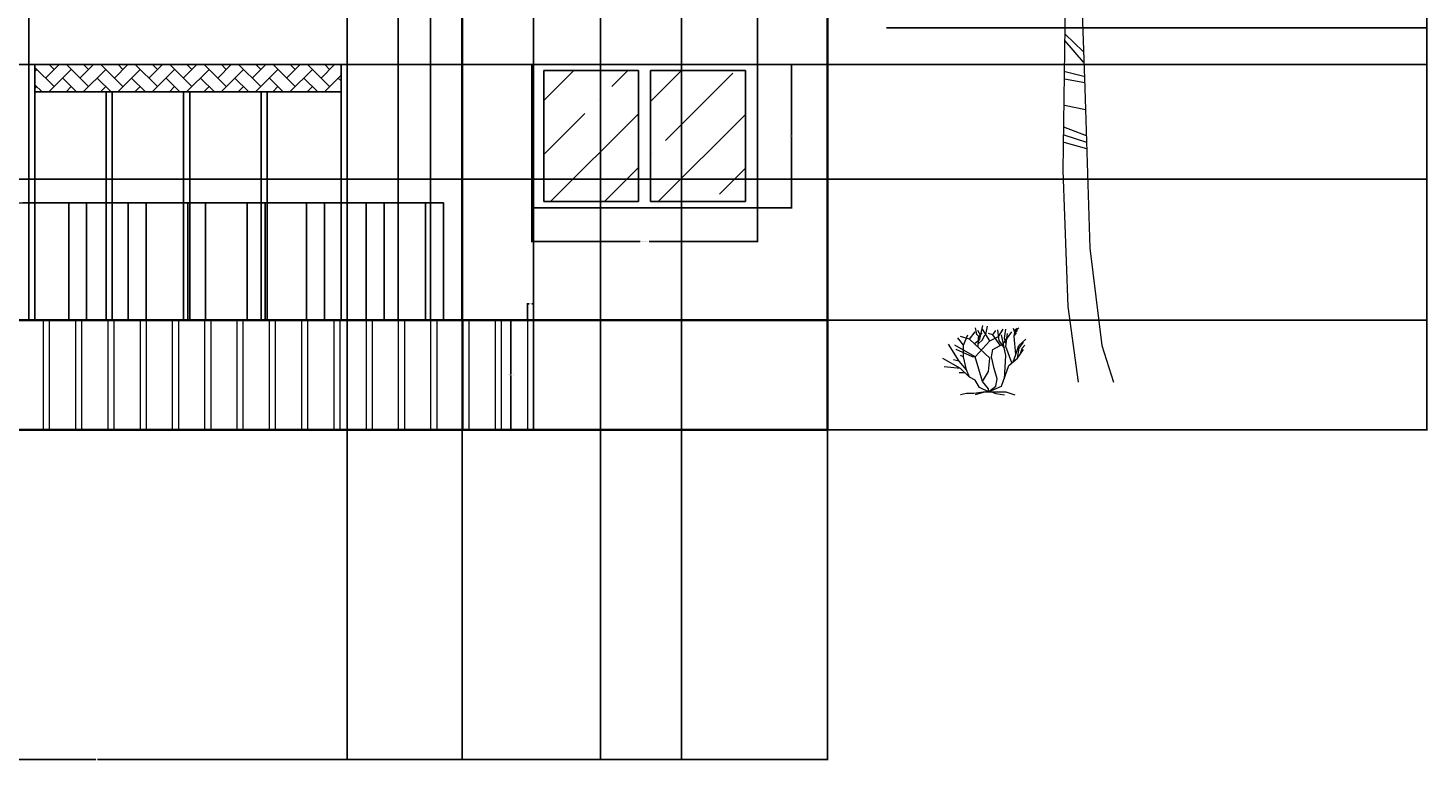
# Model space of a CAD drawing. Units: inches. Extents: x -177 to 697, y -125 to 346.
# Tile 3 of 4: x 237 to 697, y -125 to 116. Entities that reach past the tile are written whole.
import ezdxf

# ---------------------------------------------------------------- set-up
doc = ezdxf.new("R2010")
doc.units = ezdxf.units.IN
doc.header["$MEASUREMENT"] = 0
for name, color, linetype, lineweight in [('A-ANNO-DIMS', 2, 'Continuous', 18), ('A-DOOR', 3, 'Continuous', 25), ('A-FLOR-DECK', 8, 'Continuous', 18), ('A-FLOR-HRAL', 2, 'Continuous', 25), ('A-GLAZ', 4, 'Continuous', 25), ('A-GLAZ-PATT', 252, 'Continuous', 13), ('A-WALL', 7, 'Continuous', 35), ('L-PLNT', 94, 'Continuous', 13), ('S-FNDN', 7, 'Continuous', 35)]:
    doc.layers.add(name, color=color, linetype=linetype, lineweight=lineweight)
doc.styles.get("Standard").update_dxf_attribs({"font": 'arial.ttf'})
doc.dimstyles.get("Standard").update_dxf_attribs({"dimtxt": 0.18, "dimasz": 0.18, "dimexe": 0.18, "dimexo": 0.0625, "dimgap": 0.09, "dimtad": 0, "dimtih": 1, "dimtoh": 1, "dimdec": 4, "dimzin": 0, "dimdsep": 46, "dimtxsty": 'Standard', "dimcen": 0.09, "dimadec": 0, "dimazin": 0, "dimtfac": 1, "dimtdec": 4, "dimtofl": 0, "dimtmove": 0, "dimatfit": 3, "dimfxl": 1, "dimtolj": 1, "dimtzin": 0, "dimarcsym": 0})

# ---------------------------------------------------------------- blocks, each defined once
blk = doc.blocks.new('*U2')
for p, q in [((-7.5, 199.68), (-7.5, 197.946)), ((-5.567, 196.707), (-4.987, 201.167)), ((-4.407, 195.716), (-3.247, 200.672)), ((-2.474, 193.733), (-1.315, 199.433)), ((15.116, 194.477), (17.822, 198.689)), ((18.015, 195.716), (20.914, 198.689)), ((21.301, 196.459), (22.847, 198.441)), ((-20.064, 191.751), (-25.863, 193.238)), ((-15.232, 191.255), (-20.644, 193.981)), ((-9.433, 189.025), (-15.618, 193.238)), ((-6.727, 197.202), (-11.366, 197.45)), ((-3.441, 194.477), (-10.013, 195.716)), ((-1.894, 192.494), (-9.24, 193.733)), ((-1.121, 190.759), (0.232, 196.955)), ((0.038, 188.281), (1.778, 193.981)), ((5.837, 187.786), (7.577, 194.229)), ((9.317, 191.255), (10.283, 196.955)), ((11.829, 192.99), (13.182, 197.45)), ((13.956, 194.229), (14.729, 196.955)), ((14.536, 193.981), (17.242, 191.255)), ((16.082, 194.972), (17.822, 192.494)), ((18.015, 195.468), (18.981, 192.494)), ((19.368, 196.459), (19.948, 193.733)), ((20.914, 196.459), (21.301, 194.972)), ((22.074, 196.707), (23.427, 195.716)), ((23.234, 196.707), (23.62, 197.698)), ((-29.729, 190.759), (-31.469, 191.255)), ((-30.309, 190.512), (-30.695, 189.025)), ((-25.283, 191.751), (-29.342, 192.246)), ((-28.763, 190.759), (-28.763, 188.281)), ((-26.443, 191.503), (-26.636, 186.051)), ((-23.737, 191.751), (-24.51, 185.06)), ((-21.031, 191.998), (-21.804, 183.325)), ((-17.551, 191.503), (-20.451, 181.343)), ((-14.265, 190.759), (-18.131, 182.086)), ((-11.753, 189.768), (-15.425, 182.83)), ((-6.147, 186.299), (-9.24, 190.264)), ((-0.541, 189.52), (-7.307, 192.494)), ((-5.76, 190.016), (0.618, 185.308)), ((1.005, 185.803), (2.358, 190.759)), ((4.098, 185.06), (4.678, 190.512)), ((8.544, 190.512), (13.763, 189.52)), ((11.25, 192.494), (15.889, 190.512)), ((15.695, 186.299), (19.368, 188.777)), ((19.368, 187.29), (26.133, 189.768)), ((24.78, 187.538), (31.546, 188.777)), ((-8.08, 188.034), (-12.912, 182.83)), ((-4.987, 185.803), (-10.979, 182.086)), ((-5.76, 188.034), (-1.508, 182.582)), ((-2.668, 185.803), (1.198, 181.343)), ((1.005, 182.582), (2.938, 186.547)), ((4.871, 186.051), (10.09, 186.547)), ((4.871, 181.591), (8.544, 184.812)), ((6.997, 188.529), (12.216, 187.786)), ((9.51, 184.317), (15.502, 188.034)), ((11.25, 184.812), (17.628, 180.352)), ((14.536, 185.803), (19.948, 180.847)), ((17.242, 186.547), (23.041, 180.599)), ((20.721, 187.042), (25.167, 181.343)), ((23.814, 187.29), (26.907, 181.343)), ((26.133, 187.29), (29.419, 181.838)), ((28.066, 187.29), (30.966, 182.582)), ((29.806, 186.795), (32.319, 183.078)), ((29.999, 186.795), (33.092, 187.29)), ((32.512, 186.299), (35.218, 186.299)), ((33.479, 186.051), (34.445, 182.83)), ((35.605, 185.556), (37.151, 185.308)), ((35.798, 185.308), (36.958, 181.591)), ((38.118, 184.317), (38.504, 181.838)), ((-15.618, 179.36), (-20.644, 178.617)), ((-15.038, 179.36), (-10.786, 174.404)), ((-12.332, 180.104), (-9.433, 175.643)), ((-10.206, 180.104), (-8.08, 175.891)), ((-8.273, 180.104), (-6.147, 176.635)), ((-3.247, 183.821), (-8.08, 181.838)), ((-6.34, 179.608), (-4.6, 177.13)), ((-1.315, 181.591), (-5.374, 181.095)), ((-4.021, 179.36), (-2.861, 177.378)), ((-0.348, 180.352), (-1.894, 180.104)), ((2.938, 182.582), (6.61, 183.821)), ((4.098, 180.847), (8.35, 179.608)), ((5.644, 181.838), (13.569, 178.865)), ((7.384, 178.369), (10.476, 179.36)), ((7.77, 183.325), (16.082, 179.856)), ((39.857, 182.83), (40.244, 181.591)), ((-25.09, 175.148), (-28.376, 174.404)), ((-21.031, 177.626), (-24.897, 176.387)), ((-24.317, 175.891), (-18.711, 168.457)), ((-22.191, 176.635), (-16.391, 169.448)), ((-20.064, 177.626), (-15.812, 172.67)), ((-17.358, 178.617), (-13.299, 173.661)), ((-4.214, 175.148), (-14.072, 170.935)), ((-1.701, 176.882), (-8.66, 175.396)), ((-4.6, 174.9), (-4.021, 166.722)), ((-2.668, 176.387), (-2.376, 170.594)), ((-0.928, 176.882), (-1.508, 173.909)), ((2.551, 175.891), (-0.928, 171.431)), ((1.585, 177.13), (0.038, 174.652)), ((1.585, 177.13), (6.61, 176.139)), ((2.938, 175.891), (8.737, 173.413)), ((6.224, 178.121), (8.157, 175.148)), ((8.157, 178.121), (10.476, 172.422)), ((10.476, 177.874), (12.796, 169.696)), ((11.829, 177.874), (18.015, 179.113)), ((13.182, 177.874), (14.729, 166.97)), ((15.889, 177.13), (16.855, 164.492)), ((18.015, 177.13), (26.133, 179.113)), ((18.981, 175.891), (19.561, 163.005)), ((20.914, 175.891), (30.966, 176.635)), ((21.688, 175.396), (22.074, 161.518)), ((-28.956, 172.174), (-32.435, 170.192)), ((-27.409, 173.413), (-30.695, 172.67)), ((-29.922, 170.687), (-27.989, 165.235)), ((-27.989, 172.422), (-26.056, 166.227)), ((-26.829, 173.661), (-23.544, 167.218)), ((-25.476, 174.652), (-21.224, 167.466)), ((-8.466, 171.678), (-16.585, 167.713)), ((-8.853, 170.935), (-7.113, 160.527)), ((-6.92, 172.917), (-5.374, 163.253)), ((3.711, 174.404), (-0.541, 167.961)), ((5.257, 171.926), (-0.155, 163.005)), ((4.291, 173.909), (12.216, 168.953)), ((6.417, 170.439), (14.729, 164.492)), ((23.814, 174.404), (25.554, 160.279)), ((25.554, 173.661), (33.285, 173.661)), ((26.52, 173.165), (28.066, 159.784)), ((28.839, 172.174), (36.378, 170.687)), ((29.226, 171.926), (30.966, 158.545)), ((30.966, 170.687), (38.891, 167.713)), ((-32.628, 167.961), (-33.208, 167.961)), ((-32.628, 167.713), (-32.435, 165.979)), ((-31.082, 169.944), (-32.435, 169.2)), ((-31.662, 168.705), (-31.082, 165.483)), ((-12.139, 167.961), (-19.098, 162.014)), ((-12.719, 166.722), (-9.046, 154.828)), ((-10.979, 168.457), (-7.887, 157.801)), ((7.384, 168.705), (0.812, 157.553)), ((8.544, 165.979), (16.662, 160.527)), ((32.126, 169.696), (32.512, 158.545)), ((34.058, 168.705), (34.445, 158.545)), ((35.412, 167.713), (41.404, 164.988)), ((36.378, 166.474), (35.605, 158.792)), ((-14.265, 164.244), (-19.678, 158.049)), ((-14.265, 163.749), (-10.786, 154.828)), ((9.317, 164.244), (2.358, 154.332)), ((10.09, 162.51), (17.435, 157.058)), ((37.731, 165.235), (36.958, 159.288)), ((37.924, 165.235), (41.404, 163.749)), ((38.504, 164.492), (38.504, 159.536)), ((39.664, 163.253), (42.37, 161.766)), ((39.857, 162.757), (39.857, 160.031)), ((40.824, 161.766), (41.21, 160.031)), ((41.21, 161.518), (42.757, 160.279)), ((-16.005, 160.031), (-19.484, 154.084)), ((-16.585, 158.545), (-13.106, 152.35)), ((-15.618, 160.775), (-12.332, 154.332)), ((10.863, 159.784), (4.484, 152.35)), ((11.443, 157.553), (16.855, 154.332)), ((-18.131, 153.589), (-19.484, 151.606)), ((-17.938, 152.597), (-16.972, 151.111)), ((-17.358, 155.819), (-14.845, 151.358)), ((11.829, 155.075), (6.804, 150.119)), ((12.216, 153.093), (16.082, 151.606)), ((12.603, 151.111), (8.544, 148.385)), ((12.216, 148.137), (10.09, 147.393)), ((12.603, 149.872), (15.116, 149.128)), ((12.409, 145.659), (11.056, 145.659)), ((12.409, 146.898), (13.763, 146.402)), ((-4.081, 140.645), (0.753, 138.261)), ((-4.081, 137.547), (0.753, 135.163)), ((-4.081, 129.205), (1.124, 126.821)), ((-4.081, 127.298), (1.31, 123.246)), ((-4.081, 121.578), (1.31, 120.863)), ((-4.453, 112.283), (1.682, 105.133)), ((-4.267, 114.428), (1.682, 108.708)), ((-4.639, 102.273), (1.868, 100.604)), ((-4.453, 99.651), (2.24, 98.459)), ((-4.453, 91.071), (2.426, 89.641)), ((-4.825, 83.921), (2.612, 81.061)), ((-4.639, 81.299), (2.797, 78.916)), ((-4.639, 78.916), (2.797, 76.771))]:
    blk.add_line(p, q)
for points in [[(-2.363, 170.553), (-3.88, 148.505), (-4.988, 69.634), (-3.325, 24.869), (0, 0)], [(-0.116, 162.848), (0.554, 143.532), (2.217, 96.635), (3.88, 44.054), (7.76, 12.079), (11.64, 0)]]:
    blk.add_lwpolyline(points)
for centre, radius, start, end in [((-18.427, 181.448), 19.715, 350.285, 64.11229), ((25.595, 171.567), 25.395, 91.40319, 163.882), ((-21.738, 166.094), 25.899, 27.67115, 112.5305), ((23.687, 155.341), 32.188, 56.19272, 134.3213), ((-9.259, 151.732), 28.386, 68.38311, 147.5322), ((14.394, 148.393), 32.752, 113.7592, 177.4133), ((5.828, 132.718), 45.639, 35.98777, 95.82273), ((-32.8, 147.923), 45.309, 356.1943, 41.37848)]:
    blk.add_arc(centre, radius, start, end)
blk = doc.blocks.new('*U3')
for p, q in [((-16.8, 16.32), (-18.72, 18.72)), ((-14.88, 18.24), (-17.76, 19.2)), ((-16.8, 16.32), (-15.36, 19.68)), ((-14.88, 18.24), (-12.96, 20.64)), ((-12.471, 19.775), (-12.898, 22.044)), ((-11.677, 19.071), (-12.471, 19.775)), ((-11.28, 19.619), (-12.104, 21.184)), ((-12.043, 15.628), (-11.921, 18.836)), ((-11.921, 18.836), (-10.64, 20.401)), ((-11.433, 18.289), (-10.457, 22.749)), ((-10.579, 18.054), (-9.846, 19.697)), ((-8.16, 17.76), (-10.56, 21.6)), ((-9.48, 19.775), (-8.992, 22.592)), ((-7.2, 19.68), (-8.64, 20.16)), ((-8.16, 17.76), (-5.28, 19.2)), ((-7.2, 19.68), (-6.24, 21.12)), ((-4.8, 16.32), (-7.2, 19.68)), ((-5.086, 17.741), (-5.513, 21.34)), ((-5.28, 19.2), (-3.84, 21.6)), ((-2.88, 12.96), (-4.32, 19.68)), ((-3.84, 16.8), (-0.96, 20.64)), ((-3.377, 18.602), (-2.888, 21.575)), ((-2.766, 16.802), (-3.377, 18.602)), ((-2.88, 15.84), (-2.4, 20.16)), ((-0.508, 21.888), (-0.081, 20.558)), ((-0.203, 19.149), (0.102, 21.34)), ((0.346, 13.203), (-0.203, 19.149)), ((-0.142, 19.384), (0.59, 20.401)), ((-0.02, 20.01), (0.896, 21.105)), ((0.041, 20.714), (1.384, 22.044)), ((0.102, 21.34), (0.835, 21.888)), ((-18.24, 11.04), (-21.755, 16.655)), ((-12.96, 12.48), (-19.68, 16.32)), ((-13.92, 12.48), (-19.2, 14.88)), ((-16.8, 12.48), (-16.8, 16.32)), ((-8.16, 12), (-14.88, 18.24)), ((-13.325, 16.724), (-11.433, 18.289)), ((-12.96, 12.48), (-8.16, 17.76)), ((-11.982, 16.802), (-10.579, 18.054)), ((-7.68, 12.48), (-7.2, 14.88)), ((-7.2, 14.88), (-3.84, 16.8)), ((-3.377, 15.315), (-5.086, 17.819)), ((-0.96, 10.56), (-2.88, 15.84)), ((0.346, 13.203), (1.323, 16.254)), ((0.96, 12), (1.44, 15.36)), ((0.96, 12), (2.88, 14.88)), ((1.323, 16.254), (3.642, 18.289)), ((1.44, 15.36), (2.88, 17.28)), ((1.92, 13.44), (2.4, 15.36)), ((2.4, 15.36), (3.36, 16.32)), ((-17.76, 8.64), (-23.663, 11.961)), ((-17.76, 8.64), (-23.128, 9.222)), ((-18.24, 11.04), (-20.16, 11.52)), ((-15.84, 8.16), (-18.24, 11.04)), ((-16.8, 12.48), (-17.76, 12.96)), ((-15.84, 8.16), (-16.8, 12.48)), ((-12.96, 12.48), (-13.92, 12.48)), ((-10.56, 4.32), (-12.96, 12.48)), ((-8.64, 7.68), (-8.16, 12)), ((-6.72, 8.64), (-7.68, 12.48)), ((-4.32, 2.88), (-1.92, 9.6)), ((-3.36, 5.28), (-2.88, 12.96)), ((-1.92, 9.6), (0.96, 12)), ((-0.48, 10.8), (0.346, 13.203)), ((-16.32, 7.2), (-18.24, 7.2)), ((-14.88, 5.76), (-17.76, 8.64)), ((-14.88, 5.76), (-15.84, 8.16)), ((-12.96, 4.8), (-14.88, 5.76)), ((-11.52, 2.4), (-12.96, 4.8)), ((-10.56, 4.32), (-8.64, 7.68)), ((-5.76, 5.28), (-6.72, 8.64)), ((-6.24, 2.88), (-5.76, 5.28)), ((-15.84, 0.48), (-17.76, 0)), ((-13.44, 0.48), (-15.84, 0.48)), ((-9.6, 0.96), (-13.44, 0.48)), ((-9.6, 0.96), (-12.96, 0)), ((-8.64, 0.96), (-11.52, 2.4)), ((-8.64, 1.92), (-10.56, 4.32)), ((-9.6, 0.96), (-7.68, 0.96)), ((-8.64, 0.96), (-4.32, 2.88)), ((-8.64, 0.96), (-6.24, 2.88)), ((-8.64, 0.96), (-8.64, 1.92)), ((-8.64, 0.96), (-2.88, 0.96)), ((-7.68, 0.96), (-6.24, 0.48)), ((-6.24, 0.48), (-3.36, 0)), ((-2.88, 0.96), (0, 0))]:
    blk.add_line(p, q)
blk = doc.blocks.new('WIN-TWIN-LARGE-ELEV')
for p, q in [((0, 47.05), (74.16, 47.05)), ((0, 0), (0, 47.05)), ((74.16, 47.05), (74.16, 0)), ((4, 2), (4, 45.05)), ((4, 45.05), (35.01, 45.05)), ((35.01, 2), (35.01, 45.05)), ((39.01, 2), (39.01, 45.05)), ((39.01, 45.05), (70.16, 45.05)), ((70.16, 45.05), (70.16, 2)), ((74.16, 0), (0, 0)), ((35.01, 2), (4, 2)), ((70.16, 2), (39.01, 2))]:
    blk.add_line(p, q)
blk = doc.blocks.new('GUARD-POST-ELEV')
blk.add_lwpolyline([(5.89, 0), (0, 0), (0, 38.51), (5.89, 38.51)], close=True)
blk = doc.blocks.new('PORCH-UPRIGHT-36-ELEV')
for p, q in [((0, 36), (0, 0)), ((2, 36), (2, 0))]:
    blk.add_line(p, q)
blk = doc.blocks.new('*D9')
at = {"layer": 'A-ANNO-DIMS', "color": 0, "lineweight": -2, "transparency": 16777216}
for p, q in [((402.97, 56.57), (402.97, 45.33)), ((477.13, 56.57), (477.13, 45.33)), ((403.15, 45.51), (438.58, 45.51)), ((476.95, 45.51), (441.52, 45.51))]:
    blk.add_line(p, q, dxfattribs=at)
at = {"layer": 'A-ANNO-DIMS', "color": 0, "transparency": 16777216}
for points in [[(403.15, 45.54), (403.15, 45.48), (402.97, 45.51)], [(476.95, 45.54), (476.95, 45.48), (477.13, 45.51)]]:
    blk.add_solid(points, dxfattribs=at)
at = {"layer": 'Defpoints', "color": 0, "transparency": 16777216}
for p in [(402.97, 56.63), (477.13, 56.63), (477.13, 45.51)]:
    blk.add_point(p, dxfattribs=at)
at = {"layer": 'A-ANNO-DIMS', "color": 0, "transparency": 16777216, "insert": (440.05, 45.51), "char_height": 0.18, "attachment_point": 5}
blk.add_mtext('\\A1;TWIN WINDOW 74 TYP.', dxfattribs=at)
blk = doc.blocks.new('*D10')
at = {"layer": 'A-ANNO-DIMS', "color": 0, "lineweight": -2, "transparency": 16777216}
for p, q in [((477.19, 103.68), (488.44, 103.68)), ((488.26, 103.5), (488.26, 80.34)), ((488.26, 56.81), (488.26, 79.98)), ((477.19, 56.63), (488.44, 56.63))]:
    blk.add_line(p, q, dxfattribs=at)
at = {"layer": 'A-ANNO-DIMS', "color": 0, "transparency": 16777216}
for points in [[(488.23, 103.5), (488.29, 103.5), (488.26, 103.68)], [(488.23, 56.81), (488.29, 56.81), (488.26, 56.63)]]:
    blk.add_solid(points, dxfattribs=at)
at = {"layer": 'Defpoints', "color": 0, "transparency": 16777216}
for p in [(477.13, 103.68), (488.26, 103.68), (477.13, 56.63)]:
    blk.add_point(p, dxfattribs=at)
at = {"layer": 'A-ANNO-DIMS', "color": 0, "transparency": 16777216, "insert": (488.26, 80.16), "char_height": 0.18, "attachment_point": 5}
blk.add_mtext('\\A1;47 TYP.', dxfattribs=at)
blk = doc.blocks.new('*D17')
at = {"layer": 'A-ANNO-DIMS', "color": 0, "lineweight": -2, "transparency": 16777216}
for p, q in [((401.47, 19.68), (395.95, 19.68)), ((396.13, 19.5), (396.13, 1.86)), ((396.13, -16.14), (396.13, 1.5)), ((401.47, -16.32), (395.95, -16.32))]:
    blk.add_line(p, q, dxfattribs=at)
at = {"layer": 'A-ANNO-DIMS', "color": 0, "transparency": 16777216}
for points in [[(396.1, 19.5), (396.16, 19.5), (396.13, 19.68)], [(396.1, -16.14), (396.16, -16.14), (396.13, -16.32)]]:
    blk.add_solid(points, dxfattribs=at)
at = {"layer": 'Defpoints', "color": 0, "transparency": 16777216}
for p in [(396.13, 19.68), (401.53, 19.68), (401.53, -16.32)]:
    blk.add_point(p, dxfattribs=at)
at = {"layer": 'A-ANNO-DIMS', "color": 0, "transparency": 16777216, "insert": (396.13, 1.68), "char_height": 0.18, "attachment_point": 5}
blk.add_mtext('\\A1;UPRIGHT 36 TYP.', dxfattribs=at)
blk = doc.blocks.new('*D18')
at = {"layer": 'A-ANNO-DIMS', "color": 0, "lineweight": -2, "transparency": 16777216}
for p, q in [((401.53, 19.74), (401.53, 25.26)), ((401.71, 25.08), (402.07, 25.08)), ((403.35, 25.08), (402.99, 25.08)), ((403.53, 19.74), (403.53, 25.26))]:
    blk.add_line(p, q, dxfattribs=at)
at = {"layer": 'A-ANNO-DIMS', "color": 0, "transparency": 16777216}
for points in [[(401.71, 25.11), (401.71, 25.05), (401.53, 25.08)], [(403.35, 25.11), (403.35, 25.05), (403.53, 25.08)]]:
    blk.add_solid(points, dxfattribs=at)
at = {"layer": 'Defpoints', "color": 0, "transparency": 16777216}
for p in [(403.53, 25.08), (401.53, 19.68), (403.53, 19.68)]:
    blk.add_point(p, dxfattribs=at)
at = {"layer": 'A-ANNO-DIMS', "color": 0, "transparency": 16777216, "insert": (402.53, 25.08), "char_height": 0.18, "attachment_point": 5}
blk.add_mtext('\\A1;2 TYP.', dxfattribs=at)
blk = doc.blocks.new('*D19')
at = {"layer": 'A-ANNO-DIMS', "color": 0, "lineweight": -2, "transparency": 16777216}
for p, q in [((20.05, -16.38), (20.05, -124.85)), ((500.05, -16.38), (500.05, -124.85)), ((20.23, -124.67), (259.76, -124.67)), ((499.87, -124.67), (260.34, -124.67))]:
    blk.add_line(p, q, dxfattribs=at)
at = {"layer": 'A-ANNO-DIMS', "color": 0, "transparency": 16777216}
for points in [[(20.23, -124.64), (20.23, -124.7), (20.05, -124.67)], [(499.87, -124.64), (499.87, -124.7), (500.05, -124.67)]]:
    blk.add_solid(points, dxfattribs=at)
at = {"layer": 'Defpoints', "color": 0, "transparency": 16777216}
for p in [(20.05, -16.32), (500.05, -16.32), (500.05, -124.67)]:
    blk.add_point(p, dxfattribs=at)
at = {"layer": 'A-ANNO-DIMS', "color": 0, "transparency": 16777216, "insert": (260.05, -124.67), "char_height": 0.18, "attachment_point": 5}
blk.add_mtext('\\A1;480', dxfattribs=at)
blk = doc.blocks.new('*D20')
at = {"layer": 'A-ANNO-DIMS', "color": 0, "lineweight": -2, "transparency": 16777216}
for p, q in [((351.15, 306.24), (697.14, 306.24)), ((696.96, 306.06), (696.96, 145.14)), ((696.96, -16.14), (696.96, 144.78)), ((500.11, -16.32), (697.14, -16.32))]:
    blk.add_line(p, q, dxfattribs=at)
at = {"layer": 'A-ANNO-DIMS', "color": 0, "transparency": 16777216}
for points in [[(696.93, 306.06), (696.99, 306.06), (696.96, 306.24)], [(696.93, -16.14), (696.99, -16.14), (696.96, -16.32)]]:
    blk.add_solid(points, dxfattribs=at)
at = {"layer": 'Defpoints', "color": 0, "transparency": 16777216}
for p in [(351.08, 306.24), (696.96, 306.24), (500.05, -16.32)]:
    blk.add_point(p, dxfattribs=at)
at = {"layer": 'A-ANNO-DIMS', "color": 0, "transparency": 16777216, "insert": (696.96, 144.96), "char_height": 0.18, "attachment_point": 5}
blk.add_mtext('\\A1;322.56', dxfattribs=at)
blk = doc.blocks.new('*D27')
at = {"layer": 'A-ANNO-DIMS', "color": 0, "lineweight": -2, "transparency": 16777216}
for p, q in [((359.12, 19.74), (359.12, 346.22)), ((359.3, 346.04), (363.96, 346.04)), ((369.54, 346.04), (364.87, 346.04)), ((369.72, 19.74), (369.72, 346.22))]:
    blk.add_line(p, q, dxfattribs=at)
at = {"layer": 'A-ANNO-DIMS', "color": 0, "transparency": 16777216}
for points in [[(359.3, 346.07), (359.3, 346.01), (359.12, 346.04)], [(369.54, 346.07), (369.54, 346.01), (369.72, 346.04)]]:
    blk.add_solid(points, dxfattribs=at)
at = {"layer": 'Defpoints', "color": 0, "transparency": 16777216}
for p in [(359.12, 346.04), (359.12, 19.68), (369.72, 19.68)]:
    blk.add_point(p, dxfattribs=at)
at = {"layer": 'A-ANNO-DIMS', "color": 0, "transparency": 16777216, "insert": (364.42, 346.04), "char_height": 0.18, "attachment_point": 5}
blk.add_mtext('\\A1;10.604', dxfattribs=at)
blk = doc.blocks.new('*D32')
at = {"layer": 'A-ANNO-DIMS', "color": 0, "lineweight": -2, "transparency": 16777216}
for p, q in [((237.75, 103.74), (237.75, 346.22)), ((237.93, 346.04), (289.66, 346.04)), ((342.17, 346.04), (290.43, 346.04)), ((342.35, 103.74), (342.35, 346.22))]:
    blk.add_line(p, q, dxfattribs=at)
at = {"layer": 'A-ANNO-DIMS', "color": 0, "transparency": 16777216}
for points in [[(237.93, 346.07), (237.93, 346.01), (237.75, 346.04)], [(342.17, 346.07), (342.17, 346.01), (342.35, 346.04)]]:
    blk.add_solid(points, dxfattribs=at)
at = {"layer": 'Defpoints', "color": 0, "transparency": 16777216}
for p in [(342.35, 346.04), (237.75, 103.68), (342.35, 103.68)]:
    blk.add_point(p, dxfattribs=at)
at = {"layer": 'A-ANNO-DIMS', "color": 0, "transparency": 16777216, "insert": (290.05, 346.04), "char_height": 0.18, "attachment_point": 5}
blk.add_mtext('\\A1;104.6', dxfattribs=at)
blk = doc.blocks.new('*D33')
at = {"layer": 'A-ANNO-DIMS', "color": 0, "lineweight": -2, "transparency": 16777216}
for p, q in [((342.41, 103.68), (697.14, 103.68)), ((696.96, 103.5), (696.96, 61.86)), ((696.96, 19.86), (696.96, 61.5)), ((342.41, 19.68), (697.14, 19.68))]:
    blk.add_line(p, q, dxfattribs=at)
at = {"layer": 'A-ANNO-DIMS', "color": 0, "transparency": 16777216}
for points in [[(696.93, 103.5), (696.99, 103.5), (696.96, 103.68)], [(696.93, 19.86), (696.99, 19.86), (696.96, 19.68)]]:
    blk.add_solid(points, dxfattribs=at)
at = {"layer": 'Defpoints', "color": 0, "transparency": 16777216}
for p in [(342.35, 103.68), (696.96, 103.68), (342.35, 19.68)]:
    blk.add_point(p, dxfattribs=at)
at = {"layer": 'A-ANNO-DIMS', "color": 0, "transparency": 16777216, "insert": (696.96, 61.68), "char_height": 0.18, "attachment_point": 5}
blk.add_mtext('\\A1;84', dxfattribs=at)
blk = doc.blocks.new('*D35')
at = {"layer": 'A-ANNO-DIMS', "color": 0, "lineweight": -2, "transparency": 16777216}
for p, q in [((380.05, 193.5), (380.05, -124.85)), ((342.35, 167.61), (342.35, -124.85)), ((342.53, -124.67), (360.87, -124.67)), ((379.87, -124.67), (361.52, -124.67))]:
    blk.add_line(p, q, dxfattribs=at)
at = {"layer": 'A-ANNO-DIMS', "color": 0, "transparency": 16777216}
for points in [[(342.53, -124.64), (342.53, -124.7), (342.35, -124.67)], [(379.87, -124.64), (379.87, -124.7), (380.05, -124.67)]]:
    blk.add_solid(points, dxfattribs=at)
at = {"layer": 'Defpoints', "color": 0, "transparency": 16777216}
for p in [(380.05, 193.56), (342.35, 167.67), (380.05, -124.67)]:
    blk.add_point(p, dxfattribs=at)
at = {"layer": 'A-ANNO-DIMS', "color": 0, "transparency": 16777216, "insert": (361.2, -124.67), "char_height": 0.18, "attachment_point": 5}
blk.add_mtext('\\A1;37.7', dxfattribs=at)
blk = doc.blocks.new('*D37')
at = {"layer": 'A-ANNO-DIMS', "color": 0, "lineweight": -2, "transparency": 16777216}
for p, q in [((74.01, 103.68), (697.14, 103.68)), ((696.96, 103.5), (696.96, 85.05)), ((696.96, 66.24), (696.96, 84.69)), ((74.01, 66.06), (697.14, 66.06))]:
    blk.add_line(p, q, dxfattribs=at)
at = {"layer": 'A-ANNO-DIMS', "color": 0, "transparency": 16777216}
for points in [[(696.93, 103.5), (696.99, 103.5), (696.96, 103.68)], [(696.93, 66.24), (696.99, 66.24), (696.96, 66.06)]]:
    blk.add_solid(points, dxfattribs=at)
at = {"layer": 'Defpoints', "color": 0, "transparency": 16777216}
for p in [(73.94, 103.68), (696.96, 103.68), (73.94, 66.06)]:
    blk.add_point(p, dxfattribs=at)
at = {"layer": 'A-ANNO-DIMS', "color": 0, "transparency": 16777216, "insert": (696.96, 84.87), "char_height": 0.18, "attachment_point": 5}
blk.add_mtext('\\A1;37.62', dxfattribs=at)
blk = doc.blocks.new('*D40')
at = {"layer": 'A-ANNO-DIMS', "color": 0, "lineweight": -2, "transparency": 16777216}
for p, q in [((477.13, 56.7), (477.13, 346.22)), ((477.31, 346.04), (488.2, 346.04)), ((499.87, 346.04), (488.98, 346.04)), ((500.05, 19.74), (500.05, 346.22))]:
    blk.add_line(p, q, dxfattribs=at)
at = {"layer": 'A-ANNO-DIMS', "color": 0, "transparency": 16777216}
for points in [[(477.31, 346.07), (477.31, 346.01), (477.13, 346.04)], [(499.87, 346.07), (499.87, 346.01), (500.05, 346.04)]]:
    blk.add_solid(points, dxfattribs=at)
at = {"layer": 'Defpoints', "color": 0, "transparency": 16777216}
for p in [(477.13, 346.04), (477.13, 56.63), (500.05, 19.68)]:
    blk.add_point(p, dxfattribs=at)
at = {"layer": 'A-ANNO-DIMS', "color": 0, "transparency": 16777216, "insert": (488.59, 346.04), "char_height": 0.18, "attachment_point": 5}
blk.add_mtext('\\A1;22.92', dxfattribs=at)
blk = doc.blocks.new('*D41')
at = {"layer": 'A-ANNO-DIMS', "color": 0, "lineweight": -2, "transparency": 16777216}
for p, q in [((519.48, 115.68), (697.14, 115.68)), ((696.96, 115.5), (696.96, 109.86)), ((696.96, 103.86), (696.96, 109.5)), ((477.19, 103.68), (697.14, 103.68))]:
    blk.add_line(p, q, dxfattribs=at)
at = {"layer": 'A-ANNO-DIMS', "color": 0, "transparency": 16777216}
for points in [[(696.93, 115.5), (696.99, 115.5), (696.96, 115.68)], [(696.93, 103.86), (696.99, 103.86), (696.96, 103.68)]]:
    blk.add_solid(points, dxfattribs=at)
at = {"layer": 'Defpoints', "color": 0, "transparency": 16777216}
for p in [(519.41, 115.68), (477.13, 103.68), (696.96, 103.68)]:
    blk.add_point(p, dxfattribs=at)
at = {"layer": 'A-ANNO-DIMS', "color": 0, "transparency": 16777216, "insert": (696.96, 109.68), "char_height": 0.18, "attachment_point": 5}
blk.add_mtext('\\A1;12', dxfattribs=at)
blk = doc.blocks.new('*D42')
at = {"layer": 'A-ANNO-DIMS', "color": 0, "lineweight": -2, "transparency": 16777216}
for p, q in [((425.51, 190.16), (425.51, -124.85)), ((452.18, 190.16), (452.18, -124.85)), ((425.69, -124.67), (438.45, -124.67)), ((452, -124.67), (439.24, -124.67))]:
    blk.add_line(p, q, dxfattribs=at)
at = {"layer": 'A-ANNO-DIMS', "color": 0, "transparency": 16777216}
for points in [[(425.69, -124.64), (425.69, -124.7), (425.51, -124.67)], [(452, -124.64), (452, -124.7), (452.18, -124.67)]]:
    blk.add_solid(points, dxfattribs=at)
at = {"layer": 'Defpoints', "color": 0, "transparency": 16777216}
for p in [(425.51, 190.22), (452.18, 190.22), (452.18, -124.67)]:
    blk.add_point(p, dxfattribs=at)
at = {"layer": 'A-ANNO-DIMS', "color": 0, "transparency": 16777216, "insert": (438.84, -124.67), "char_height": 0.18, "attachment_point": 5}
blk.add_mtext('\\A1;26.67', dxfattribs=at)
blk = doc.blocks.new('*D50')
at = {"layer": 'A-ANNO-DIMS', "color": 0, "lineweight": -2, "transparency": 16777216}
for p, q in [((403.53, -16.26), (403.53, 346.22)), ((403.71, 346.04), (451.4, 346.04)), ((499.87, 346.04), (452.18, 346.04)), ((500.05, -16.26), (500.05, 346.22))]:
    blk.add_line(p, q, dxfattribs=at)
at = {"layer": 'A-ANNO-DIMS', "color": 0, "transparency": 16777216}
for points in [[(403.71, 346.07), (403.71, 346.01), (403.53, 346.04)], [(499.87, 346.07), (499.87, 346.01), (500.05, 346.04)]]:
    blk.add_solid(points, dxfattribs=at)
at = {"layer": 'Defpoints', "color": 0, "transparency": 16777216}
for p in [(500.05, 346.04), (403.53, -16.32), (500.05, -16.32)]:
    blk.add_point(p, dxfattribs=at)
at = {"layer": 'A-ANNO-DIMS', "color": 0, "transparency": 16777216, "insert": (451.79, 346.04), "char_height": 0.18, "attachment_point": 5}
blk.add_mtext('\\A1;96.52', dxfattribs=at)

msp = doc.modelspace()

# ---------------------------------------------------------------- hatches: boundary and pattern name
at = {"layer": 'A-GLAZ-PATT'}
h = msp.add_hatch(dxfattribs=at)
h.set_pattern_fill('AR-HBONE', color=256)
h.set_pattern_definition([(45, (-118.808, -115.7344), (0, 5.656854), [12, -4]), (135, (-115.9797, -112.906), (4e-16, 5.656854), [12, -4])])
h.paths.add_polyline_path([(340.3468, 223.6802), (239.7524, 223.6802), (239.7524, 214.6802), (340.3468, 214.6802)])
h.paths.add_polyline_path([(340.3468, 103.6802), (239.7524, 103.6802), (239.7524, 94.6802), (340.3468, 94.6802)])
h = msp.add_hatch(dxfattribs=at)
h.set_pattern_fill('ANSI35', color=256, scale=100)
h.set_pattern_definition([(45, (-118.808, -115.734), (-17.6777, 17.6777), []), (45, (-101.13, -115.734), (-17.6777, 17.6777), [31.25, -6.25, 0, -6.25])])
h.paths.add_polyline_path([(437.9807, 101.6802), (406.9675, 101.6802), (406.9675, 58.6343), (437.9807, 58.6343)])
h.paths.add_polyline_path([(473.1317, 101.6802), (441.9807, 101.6802), (441.9807, 58.6343), (473.1317, 58.6343)])

# ---------------------------------------------------------------- linework, layer by layer
at = {"layer": 'A-DOOR'}
for p, q in [((342.3468, 103.6802), (237.7524, 103.6802)), ((237.7524, 103.6802), (237.7524, 19.6802)), ((239.7524, 103.6802), (239.7524, 19.6802)), ((340.3468, 19.6802), (340.3468, 103.6802)), ((342.3468, 19.6802), (342.3468, 103.6802)), ((340.3468, 94.6802), (239.7524, 94.6802)), ((263.1757, 94.6802), (263.1757, 19.6802)), ((265.1757, 94.6802), (265.1757, 19.6802)), ((288.5989, 94.6802), (288.5989, 19.6802)), ((290.5989, 94.6802), (290.5989, 19.6802)), ((314.0222, 94.6802), (314.0222, 19.6802)), ((316.0222, 94.6802), (316.0222, 19.6802)), ((237.7524, 19.6802), (342.3468, 19.6802))]:
    msp.add_line(p, q, dxfattribs=at)
at = {"layer": 'A-FLOR-HRAL'}
msp.add_open_spline([(133.4757, 28.1928), (141.2082, 32.2346), (156.9836, 40.4804), (177.8872, 50.6849), (196.9965, 59.8479), (216.4528, 57.5999), (235.2353, 58.3169), (254.7984, 58.158), (273.345, 58.2027), (293.4178, 58.1899), (312.9537, 58.1935), (332.4903, 58.1926), (351.4925, 58.1928), (364.5168, 58.1928), (371.029, 58.1928)], degree=3, knots=[0, 0, 0, 0, 26.12758735, 53.30341094, 70.42401933, 88.05900671, 110.54286492, 127.13195594, 146.66843056, 166.20490518, 187.34399835, 205.27785442, 224.81432904, 244.35080366, 244.35080366, 244.35080366, 244.35080366], dxfattribs=at)
at = {"layer": 'A-WALL'}
for p, q in [((380.0496, 19.6802), (380.0496, 235.6802)), ((500.0496, 235.6802), (500.0496, -16.3198))]:
    msp.add_line(p, q, dxfattribs=at)
at = {"layer": 'S-FNDN'}
for p, q in [((20.0496, 19.6802), (500.0496, 19.6802)), ((500.0496, -16.3198), (20.0496, -16.3198))]:
    msp.add_line(p, q, dxfattribs=at)

# ---------------------------------------------------------------- block references
at = {"layer": 'A-FLOR-DECK'}
for p in [(242.4673, -16.3198), (253.0717, -16.3198), (263.6761, -16.3198), (274.2806, -16.3198), (284.885, -16.3198), (295.4894, -16.3198), (306.0939, -16.3198), (316.6983, -16.3198), (327.3027, -16.3198), (337.9071, -16.3198), (348.5116, -16.3198), (359.116, -16.3198), (369.7204, -16.3198), (380.3248, -16.3198), (390.9293, -16.3198), (401.5337, -16.3198)]:
    msp.add_blockref('PORCH-UPRIGHT-36-ELEV', p, dxfattribs=at)
at = {"layer": 'A-FLOR-HRAL'}
for p in [(250.8628, 19.6802), (270.3992, 19.6802), (289.9357, 19.6802), (309.4722, 19.6802), (329.0087, 19.6802), (348.5451, 19.6802), (368.0816, 19.6802)]:
    msp.add_blockref('GUARD-POST-ELEV', p, dxfattribs=at)
at = {"layer": 'A-GLAZ'}
msp.add_blockref('WIN-TWIN-LARGE-ELEV', (402.9675, 56.6343), dxfattribs=at)
at = {"layer": 'L-PLNT'}
for name, p in [('*U2', (582.3957, -0.7305)), ('*U3', (561.59, -4.851))]:
    msp.add_blockref(name, p, dxfattribs=at)

# ---------------------------------------------------------------- dimensions: what is measured, and where the dimension line sits
at = {"layer": 'A-ANNO-DIMS'}
for base, p1, p2, override, picture, middle in [((342.3468, 346.0391), (237.7524, 103.6802), (342.3468, 103.6802), {"dimdec": 1, "dimlfac": 1, "dimrnd": 0, "dimzin": 0, "dimdsep": 46, "dimlunit": 2}, '*D32', (290.0496, 346.0391)), ((359.116, 346.0391), (369.7204, 19.6802), (359.116, 19.6802), {"dimdec": 3, "dimlfac": 1, "dimrnd": 0, "dimzin": 0, "dimdsep": 46, "dimlunit": 2}, '*D27', (364.4182, 346.0391)), ((500.0496, 346.0391), (403.5337, -16.3198), (500.0496, -16.3198), {"dimdec": 2, "dimlfac": 1, "dimrnd": 0, "dimzin": 0, "dimdsep": 46, "dimlunit": 2}, '*D50', (451.7916, 346.0391)), ((477.1317, 346.0391), (500.0496, 19.6802), (477.1317, 56.6343), {"dimdec": 2, "dimlfac": 1, "dimrnd": 0, "dimzin": 0, "dimdsep": 46, "dimlunit": 2}, '*D40', (488.5906, 346.0391)), ((380.0496, -124.671), (342.3468, 167.6715), (380.0496, 193.5592), {"dimdec": 1, "dimlfac": 1, "dimrnd": 0, "dimzin": 0, "dimdsep": 46, "dimlunit": 2}, '*D35', (361.1982, -124.671)), ((452.1768, -124.671), (425.5056, 190.2226), (452.1768, 190.2226), {"dimdec": 2, "dimlfac": 1, "dimrnd": 0, "dimzin": 0, "dimdsep": 46, "dimlunit": 2}, '*D42', (438.8412, -124.671)), ((500.0496, -124.671), (20.0496, -16.3198), (500.0496, -16.3198), {"dimdec": 0, "dimlfac": 1, "dimrnd": 0, "dimzin": 0, "dimdsep": 46, "dimlunit": 2}, '*D19', (260.0496, -124.671))]:
    dim = msp.add_linear_dim(base=base, p1=p1, p2=p2, dimstyle='Standard', override=override, dxfattribs=at)
    dim.commit()
    dim.dimension.update_dxf_attribs({"geometry": picture, "text_midpoint": middle})
for base, p1, p2, override, picture, middle in [((696.9617, 306.2391), (500.0496, -16.3198), (351.0833, 306.2391), {"dimdec": 2, "dimlfac": 1, "dimrnd": 0, "dimzin": 0, "dimdsep": 46, "dimlunit": 2}, '*D20', (696.9617, 144.9597)), ((696.9617, 103.6802), (519.4137, 115.6802), (477.1317, 103.6802), {"dimdec": 0, "dimlfac": 1, "dimrnd": 0, "dimzin": 0, "dimdsep": 46, "dimlunit": 2}, '*D41', (696.9617, 109.6802)), ((696.9617, 103.6802), (73.9429, 66.059), (73.9429, 103.6802), {"dimdec": 2, "dimlfac": 1, "dimrnd": 0, "dimzin": 0, "dimdsep": 46, "dimlunit": 2}, '*D37', (696.9617, 84.8696)), ((696.9617, 103.6802), (342.3468, 19.6802), (342.3468, 103.6802), {"dimdec": 0, "dimlfac": 1, "dimrnd": 0, "dimzin": 0, "dimdsep": 46, "dimlunit": 2}, '*D33', (696.9617, 61.6802))]:
    dim = msp.add_linear_dim(base=base, p1=p1, p2=p2, angle=90, dimstyle='Standard', override=override, dxfattribs=at)
    dim.commit()
    dim.dimension.update_dxf_attribs({"geometry": picture, "text_midpoint": middle})
for base, p1, p2, text, picture, middle in [((488.2563, 103.6802), (477.1317, 56.6343), (477.1317, 103.6802), '<> TYP.', '*D10', (488.2563, 80.1573)), ((396.1337, 19.6802), (401.5337, -16.3198), (401.5337, 19.6802), 'UPRIGHT <> TYP.', '*D17', (396.1337, 1.6802))]:
    dim = msp.add_linear_dim(base=base, p1=p1, p2=p2, angle=90, text=text, dimstyle='Standard', override={"dimdec": 0, "dimlfac": 1, "dimrnd": 0, "dimzin": 0, "dimdsep": 46, "dimlunit": 2}, dxfattribs=at)
    dim.commit()
    dim.dimension.update_dxf_attribs({"geometry": picture, "text_midpoint": middle})
for base, p1, p2, text, picture, middle in [((477.1317, 45.5096), (402.9675, 56.6343), (477.1317, 56.6343), 'TWIN WINDOW <> TYP.', '*D9', (440.0496, 45.5096)), ((403.5337, 25.0802), (401.5337, 19.6802), (403.5337, 19.6802), '<> TYP.', '*D18', (402.5337, 25.0802))]:
    dim = msp.add_linear_dim(base=base, p1=p1, p2=p2, text=text, dimstyle='Standard', override={"dimdec": 0, "dimlfac": 1, "dimrnd": 0, "dimzin": 0, "dimdsep": 46, "dimlunit": 2}, dxfattribs=at)
    dim.commit()
    dim.dimension.update_dxf_attribs({"geometry": picture, "text_midpoint": middle})

doc.saveas('drawing.dxf')
